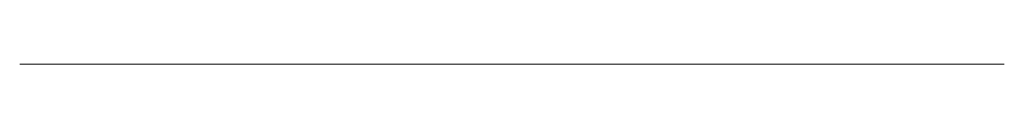
# Model space of a CAD drawing. Units: millimetres. Extents: x 527.79 to 532.79, y 595.7 to 595.7.
import ezdxf

# ---------------------------------------------------------------- set-up
doc = ezdxf.new("R2010")
doc.units = ezdxf.units.MM
doc.layers.add('M-CONS', color=8, linetype='Continuous', lineweight=13)

msp = doc.modelspace()

# ---------------------------------------------------------------- linework, layer by layer
at = {"layer": 'M-CONS'}
msp.add_line((527.7889, 595.7001, 90), (532.7889, 595.7001, 90), dxfattribs=at)

doc.saveas('drawing.dxf')
